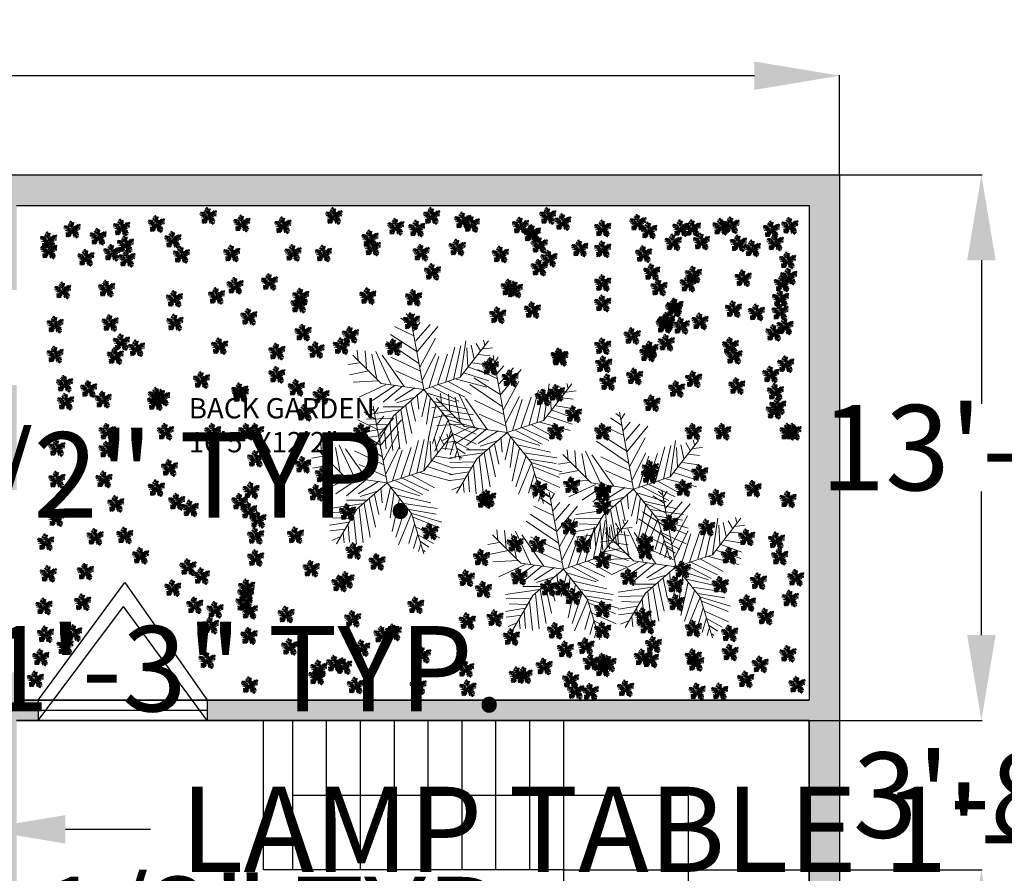
# Model space of a CAD drawing. Units: inches. Extents: x 23 to 3024, y 4 to 1405.
# Tile 6 of 7: x 2558 to 2849, y 1090 to 1342. Entities that reach past the tile are written whole.
import ezdxf

# ---------------------------------------------------------------- set-up
doc = ezdxf.new("R2010")
doc.units = ezdxf.units.IN
doc.header["$MEASUREMENT"] = 0
for name, color, linetype, lineweight in [('A-ANNO-DIMS', 2, 'Continuous', 18), ('A-DOOR', 4, 'Continuous', 25), ('A-FLOR-STRS', 7, 'Continuous', 25), ('A-WALL', 7, 'Continuous', 35), ('A-WALL-PATT', 189, 'Continuous', 13), ('C-PROP', 7, 'Continuous', 30), ('L-PLNT', 114, 'Continuous', 13)]:
    doc.layers.add(name, color=color, linetype=linetype, lineweight=lineweight)
doc.layers.add('A-AREA-IDEN', color=30, linetype='Continuous', lineweight=18, true_color=0xf8991e)
doc.styles.get("Standard").update_dxf_attribs({"font": 'arial.ttf'})
doc.dimstyles.get("Standard").update_dxf_attribs({"dimtxt": 25.18, "dimasz": 25.18, "dimexe": 0.18, "dimexo": 0.0625, "dimgap": 0.09, "dimtad": 0, "dimtih": 1, "dimtoh": 1, "dimdec": 0, "dimrnd": 10, "dimzin": 0, "dimdsep": 46, "dimlunit": 3, "dimtxsty": 'Standard', "dimcen": 0.09, "dimadec": 0, "dimazin": 0, "dimtfac": 1, "dimtdec": 0, "dimtofl": 0, "dimtmove": 0, "dimatfit": 3, "dimfxl": 1, "dimtolj": 1, "dimtzin": 0, "dimarcsym": 0})

# ---------------------------------------------------------------- blocks, each defined once
blk = doc.blocks.new('*U8')
for p, q in [((-8.737, 47.138), (-17.069, 52.711)), ((-10.186, 53.64), (-13.084, 55.962)), ((0, 0), (-10.5, 57)), ((-9.099, 51.782), (-6.563, 55.962)), ((-7.288, 39.707), (-21.778, 46.673)), ((-7.65, 43.423), (-2.578, 49.46)), ((-5.839, 35.992), (4.667, 48.067)), ((-5.114, 27.632), (10.463, 46.673)), ((-5.114, 28.097), (-24.676, 40.636)), ((-2.941, 16.486), (8.652, 37.85)), ((-3.665, 19.273), (-27.574, 35.527)), ((16.259, 5.805), (23.142, 31.348)), ((22.055, 7.198), (27.489, 32.277)), ((27, 9), (48, 36)), ((27.127, 9.056), (31.112, 35.992)), ((31.836, 30.883), (32.561, 16.486)), ((35.096, 32.741), (37.27, 22.524)), ((38.719, 34.134), (41.979, 28.561)), ((43.791, 29.954), (51.036, 30.883)), ((44.153, 36.456), (45.239, 32.741)), ((-31.5, 4.5), (-52.5, 25.5)), ((-48.585, 21.131), (-49.309, 29.026)), ((-43.513, 28.561), (-42.427, 15.558)), ((-38.442, 26.239), (-34.819, 7.663)), ((-35.544, 28.097), (-24.314, 3.947)), ((-14.533, 2.09), (-30.834, 25.31)), ((-24.314, 23.917), (-2.941, 13.7)), ((-1.129, 6.734), (9.014, 26.704)), ((3.942, 1.625), (11.187, 24.381)), ((10.101, 3.483), (17.708, 26.239)), ((40.53, 25.775), (48.862, 24.846)), ((-47.498, 19.737), (-55.83, 18.344)), ((33.285, 16.486), (48.862, 10.913)), ((36.183, 19.737), (48.137, 17.88)), ((-40.615, 13.7), (-55.105, 10.913)), ((-20.691, 13.7), (-1.129, 4.876)), ((0, 0), (27, 9)), ((24.229, 7.663), (46.688, 1.625)), ((29.662, 12.307), (48.137, 6.269)), ((-33.37, 6.269), (-52.207, 5.34)), ((-28.299, 3.483), (-47.86, -5.805)), ((-21.416, 3.018), (-38.079, -8.128)), ((0, 0), (-31.5, 4.5)), ((-15.982, 2.09), (-30.11, -9.521)), ((0, 0), (-22.5, -19.5)), ((-6.563, 1.161), (-21.416, -8.128)), ((0, 0), (18, -22.5)), ((6.478, 1.625), (26.04, -8.592)), ((11.187, 3.483), (30.749, -5.805)), ((18.07, 5.805), (35.096, -3.483)), ((-6.563, -5.805), (-19.967, -9.985)), ((-4.752, -3.483), (-3.665, -14.629)), ((2.493, -3.019), (-1.491, -20.202)), ((1.769, -2.555), (24.229, -9.521)), ((5.029, -6.27), (2.131, -25.775)), ((-15.257, -12.772), (-30.11, -12.772)), ((-13.446, -11.378), (-8.737, -32.741)), ((-9.461, -8.592), (-6.201, -23.453)), ((9.014, -11.378), (3.58, -35.992)), ((7.565, -9.056), (32.198, -14.629)), ((-17.431, -15.094), (-42.789, -18.809)), ((-24.314, -21.596), (-42.427, -22.06)), ((-22.5, -19.5), (-37.5, -45)), ((-20.691, -18.345), (-17.793, -44.352)), ((-17.069, -15.094), (-12.721, -40.172)), ((14.085, -16.951), (6.478, -40.172)), ((12.274, -15.094), (36.907, -18.809)), ((16.259, -19.738), (36.183, -22.989)), ((-28.299, -29.026), (-42.789, -31.348)), ((-26.849, -26.24), (-40.253, -25.775)), ((-25.038, -23.918), (-22.865, -45.281)), ((18.07, -22.524), (8.289, -45.745)), ((18, -22.5), (27, -52.5)), ((18.433, -22.524), (40.53, -29.026)), ((19.157, -25.311), (38.719, -33.206)), ((-30.834, -34.135), (-42.427, -35.528)), ((-29.023, -30.884), (-27.936, -43.887)), ((20.244, -30.419), (15.897, -44.816)), ((21.331, -32.741), (39.081, -40.636)), ((-34.457, -39.708), (-40.978, -42.494)), ((-32.646, -36.921), (-31.921, -44.352)), ((22.78, -37.85), (19.519, -48.532)), ((22.78, -38.314), (34.372, -44.816)), ((24.591, -43.423), (30.749, -47.603)), ((24.591, -45.745), (23.142, -50.854)), ((26.764, -49.925), (28.213, -50.854))]:
    blk.add_line(p, q)
blk = doc.blocks.new('*D9')
at = {"layer": 'A-ANNO-DIMS', "color": 0, "lineweight": -2, "transparency": 16777216}
for p, q in [((2200.45, 1295.99), (2200.45, 1325.4)), ((2225.63, 1325.22), (2478.99, 1325.22)), ((2775.27, 1325.22), (2521.91, 1325.22)), ((2800.45, 1295.99), (2800.45, 1325.4))]:
    blk.add_line(p, q, dxfattribs=at)
at = {"layer": 'A-ANNO-DIMS', "color": 0, "transparency": 16777216}
for points in [[(2225.63, 1329.42), (2225.63, 1321.02), (2200.45, 1325.22)], [(2775.27, 1329.42), (2775.27, 1321.02), (2800.45, 1325.22)]]:
    blk.add_solid(points, dxfattribs=at)
at = {"layer": 'Defpoints', "color": 0, "transparency": 16777216}
for p in [(2800.45, 1325.22), (2200.45, 1295.93), (2800.45, 1295.93)]:
    blk.add_point(p, dxfattribs=at)
at = {"layer": 'A-ANNO-DIMS', "color": 0, "transparency": 16777216, "insert": (2500.45, 1325.22), "char_height": 25.18, "attachment_point": 5}
blk.add_mtext("\\A1;50'", dxfattribs=at)
blk = doc.blocks.new('*D25')
at = {"layer": 'A-ANNO-DIMS', "color": 0, "lineweight": -2, "transparency": 16777216}
for p, q in [((2273.17, 1211.86), (2273.17, 1207.21)), ((2303.45, 1211.86), (2303.45, 1207.21)), ((2247.99, 1207.39), (2222.81, 1207.39)), ((2328.63, 1207.39), (2353.81, 1207.39))]:
    blk.add_line(p, q, dxfattribs=at)
at = {"layer": 'A-ANNO-DIMS', "color": 0, "transparency": 16777216}
for points in [[(2247.99, 1211.58), (2247.99, 1203.19), (2273.17, 1207.39)], [(2328.63, 1211.58), (2328.63, 1203.19), (2303.45, 1207.39)]]:
    blk.add_solid(points, dxfattribs=at)
at = {"layer": 'Defpoints', "color": 0, "transparency": 16777216}
for p in [(2273.17, 1211.93), (2303.45, 1211.93), (2303.45, 1207.39)]:
    blk.add_point(p, dxfattribs=at)
at = {"layer": 'A-ANNO-DIMS', "color": 0, "transparency": 16777216, "insert": (2517, 1207.39), "char_height": 25.18, "attachment_point": 5}
blk.add_mtext('\\A1;DOOR 2\'-6 1/2" TYP.', dxfattribs=at)
blk = doc.blocks.new('*D37')
at = {"layer": 'A-ANNO-DIMS', "color": 0, "lineweight": -2, "transparency": 16777216}
for p, q in [((2214.42, 1078.46), (2214.42, 1076)), ((2230.01, 1078.46), (2230.01, 1076)), ((2189.24, 1076.18), (2164.06, 1076.18)), ((2255.19, 1076.18), (2280.37, 1076.18))]:
    blk.add_line(p, q, dxfattribs=at)
at = {"layer": 'A-ANNO-DIMS', "color": 0, "transparency": 16777216}
for points in [[(2189.24, 1080.38), (2189.24, 1071.99), (2214.42, 1076.18)], [(2255.19, 1080.38), (2255.19, 1071.99), (2230.01, 1076.18)]]:
    blk.add_solid(points, dxfattribs=at)
at = {"layer": 'Defpoints', "color": 0, "transparency": 16777216}
for p in [(2214.42, 1078.52), (2230.01, 1078.52), (2230.01, 1076.18)]:
    blk.add_point(p, dxfattribs=at)
at = {"layer": 'A-ANNO-DIMS', "color": 0, "transparency": 16777216, "insert": (2499.37, 1076.18), "char_height": 25.18, "attachment_point": 5}
blk.add_mtext('\\A1;LAMP TABLE 1\'-3 1/2" TYP.', dxfattribs=at)
blk = doc.blocks.new('*D39')
at = {"layer": 'A-ANNO-DIMS', "color": 0, "lineweight": -2, "transparency": 16777216}
for p, q in [((2501.85, 1102.79), (2476.67, 1102.79)), ((2527.03, 1099.9), (2527.03, 1102.97)), ((2546.68, 1099.9), (2546.68, 1102.97)), ((2571.86, 1102.79), (2597.04, 1102.79))]:
    blk.add_line(p, q, dxfattribs=at)
at = {"layer": 'A-ANNO-DIMS', "color": 0, "transparency": 16777216}
for points in [[(2501.85, 1106.99), (2501.85, 1098.59), (2527.03, 1102.79)], [(2571.86, 1106.99), (2571.86, 1098.59), (2546.68, 1102.79)]]:
    blk.add_solid(points, dxfattribs=at)
at = {"layer": 'Defpoints', "color": 0, "transparency": 16777216}
for p in [(2546.68, 1102.79), (2527.03, 1099.84), (2546.68, 1099.84)]:
    blk.add_point(p, dxfattribs=at)
at = {"layer": 'A-ANNO-DIMS', "color": 0, "transparency": 16777216, "insert": (2816.04, 1102.79), "char_height": 25.18, "attachment_point": 5}
blk.add_mtext('\\A1;LAMP TABLE 1\'-7 1/2" TYP.', dxfattribs=at)
blk = doc.blocks.new('*D40')
at = {"layer": 'A-ANNO-DIMS', "color": 0, "lineweight": -2, "transparency": 16777216}
for p, q in [((2524.09, 1125.02), (2524.09, 1150.2)), ((2524.09, 1150.2), (2549.27, 1150.2)), ((2526.97, 1099.84), (2523.91, 1099.84)), ((2526.97, 1084.82), (2523.91, 1084.82)), ((2524.09, 1059.64), (2524.09, 1034.46))]:
    blk.add_line(p, q, dxfattribs=at)
at = {"layer": 'A-ANNO-DIMS', "color": 0, "transparency": 16777216}
for points in [[(2519.89, 1125.02), (2528.28, 1125.02), (2524.09, 1099.84)], [(2519.89, 1059.64), (2528.28, 1059.64), (2524.09, 1084.82)]]:
    blk.add_solid(points, dxfattribs=at)
at = {"layer": 'Defpoints', "color": 0, "transparency": 16777216}
for p in [(2524.09, 1099.84), (2527.03, 1099.84), (2527.03, 1084.82)]:
    blk.add_point(p, dxfattribs=at)
at = {"layer": 'A-ANNO-DIMS', "color": 0, "transparency": 16777216, "insert": (2624.91, 1150.2), "char_height": 25.18, "attachment_point": 5}
blk.add_mtext('\\A1;1\'-3" TYP.', dxfattribs=at)
blk = doc.blocks.new('*D43')
at = {"layer": 'A-ANNO-DIMS', "color": 0, "lineweight": -2, "transparency": 16777216}
for p, q in [((2800.51, 1295.93), (2842.48, 1295.93)), ((2842.3, 1270.75), (2842.3, 1228.38)), ((2842.3, 1160.11), (2842.3, 1202.47)), ((2791.51, 1134.93), (2842.48, 1134.93))]:
    blk.add_line(p, q, dxfattribs=at)
at = {"layer": 'A-ANNO-DIMS', "color": 0, "transparency": 16777216}
for points in [[(2838.1, 1270.75), (2846.5, 1270.75), (2842.3, 1295.93)], [(2838.1, 1160.11), (2846.5, 1160.11), (2842.3, 1134.93)]]:
    blk.add_solid(points, dxfattribs=at)
at = {"layer": 'Defpoints', "color": 0, "transparency": 16777216}
for p in [(2800.45, 1295.93), (2791.45, 1134.93), (2842.3, 1134.93)]:
    blk.add_point(p, dxfattribs=at)
at = {"layer": 'A-ANNO-DIMS', "color": 0, "transparency": 16777216, "insert": (2842.3, 1215.43), "char_height": 25.18, "attachment_point": 5}
blk.add_mtext('\\A1;13\'-5"', dxfattribs=at)
blk = doc.blocks.new('*D46')
at = {"layer": 'A-ANNO-DIMS', "color": 0, "lineweight": -2, "transparency": 16777216}
for p, q in [((2719.07, 1090.84), (2842.48, 1090.84)), ((2842.3, 1065.66), (2842.3, 1052.75)), ((2842.3, 1013.96), (2842.3, 1026.86)), ((2791.51, 988.78), (2842.48, 988.78))]:
    blk.add_line(p, q, dxfattribs=at)
at = {"layer": 'A-ANNO-DIMS', "color": 0, "transparency": 16777216}
for points in [[(2838.1, 1065.66), (2846.5, 1065.66), (2842.3, 1090.84)], [(2838.1, 1013.96), (2846.5, 1013.96), (2842.3, 988.78)]]:
    blk.add_solid(points, dxfattribs=at)
at = {"layer": 'Defpoints', "color": 0, "transparency": 16777216}
for p in [(2719, 1090.84), (2842.3, 1090.84), (2791.45, 988.78)]:
    blk.add_point(p, dxfattribs=at)
at = {"layer": 'A-ANNO-DIMS', "color": 0, "transparency": 16777216, "insert": (2842.3, 1039.81), "char_height": 25.18, "attachment_point": 5}
blk.add_mtext('\\A1;8\'-6"', dxfattribs=at)
blk = doc.blocks.new('*D47')
at = {"layer": 'A-ANNO-DIMS', "color": 0, "lineweight": -2, "transparency": 16777216}
for p, q in [((2842.3, 1160.11), (2842.3, 1185.29)), ((2719.07, 1134.93), (2842.48, 1134.93)), ((2719.07, 1090.84), (2842.48, 1090.84)), ((2842.3, 1065.66), (2842.3, 1040.48))]:
    blk.add_line(p, q, dxfattribs=at)
at = {"layer": 'A-ANNO-DIMS', "color": 0, "transparency": 16777216}
for points in [[(2838.1, 1160.11), (2846.5, 1160.11), (2842.3, 1134.93)], [(2838.1, 1065.66), (2846.5, 1065.66), (2842.3, 1090.84)]]:
    blk.add_solid(points, dxfattribs=at)
at = {"layer": 'Defpoints', "color": 0, "transparency": 16777216}
for p in [(2719, 1134.93), (2842.3, 1134.93), (2719, 1090.84)]:
    blk.add_point(p, dxfattribs=at)
at = {"layer": 'A-ANNO-DIMS', "color": 0, "transparency": 16777216, "insert": (2842.3, 1112.88), "char_height": 25.18, "attachment_point": 5}
blk.add_mtext('\\A1;3\'-8"', dxfattribs=at)

msp = doc.modelspace()

# ---------------------------------------------------------------- hatches: boundary and pattern name
at = {"layer": 'A-WALL-PATT'}
h = msp.add_hatch(color=256, dxfattribs=at)
h.dxf.hatch_style = 1
h.paths.add_polyline_path([(2209.45, 1233.93), (2200.45, 1233.93), (2200.45, 1160.43), (2209.45, 1160.43), (2209.45, 1167.77), (2209.45, 1202.93), (2306.45, 1202.93), (2306.45, 1208.93), (2300.45, 1208.93), (2209.45, 1208.93)], flags=17)
h.paths.add_polyline_path([(2800.45, 1295.93), (2200.45, 1295.93), (2160.45, 1295.93), (2160.45, 575.93), (2200.45, 575.93), (2228.06, 575.93), (2228.06, 584.93), (2209.45, 584.93), (2209.45, 856.93), (2200.45, 856.93), (2200.45, 581.93), (2166.45, 581.93), (2166.45, 1289.93), (2200.45, 1289.93), (2200.45, 1261.93), (2209.45, 1261.93), (2209.45, 1286.93), (2244.45, 1286.93), (2300.45, 1286.93), (2300.45, 1241.93), (2301.45, 1241.93, -0.017236), (2303.45, 1241.93), (2306.45, 1241.93), (2306.45, 1286.93), (2548.45, 1286.93), (2548.45, 1261.93), (2557.45, 1261.93), (2557.45, 1286.93), (2791.45, 1286.93), (2791.45, 1140.93), (2613.74, 1140.93), (2613.74, 1134.93), (2791.45, 1134.93), (2791.45, 927.1), (2800.45, 927.1)])
h.paths.add_polyline_path([(2166.06, 1284.53), (2166.03, 1284.87), (2166.29, 1284.91), (2166.32, 1284.58)], flags=16)
h.paths.add_polyline_path([(2557.45, 1233.93), (2548.45, 1233.93), (2548.45, 1208.93), (2514.78, 1208.93), (2457.45, 1208.93), (2451.45, 1208.93), (2451.45, 1202.93), (2548.45, 1202.93), (2557.45, 1202.93)], flags=17)
h.paths.add_polyline_path([(2457.45, 1286.93), (2451.45, 1286.93), (2451.45, 1241.93), (2454.45, 1241.93, -0.017236), (2456.45, 1241.93), (2457.45, 1241.93)], flags=17)
h.paths.add_polyline_path([(2419.96, 1208.93), (2378.45, 1208.93), (2378.45, 1286.93), (2372.45, 1286.93), (2372.45, 1208.93), (2352.45, 1208.93), (2352.45, 1202.93), (2419.96, 1202.93)], flags=17)
h.paths.add_polyline_path([(2557.45, 1134.93), (2563.84, 1134.93), (2563.84, 1140.93), (2557.45, 1140.93), (2557.45, 1149.12), (2548.45, 1149.12), (2548.45, 1103.07), (2548.45, 1065.93), (2416.45, 1065.93), (2416.45, 1064.93, -0.014283), (2416.45, 1062.93), (2416.45, 1059.93), (2548.45, 1059.93), (2548.45, 1025.12), (2557.45, 1025.12)], flags=17)
h.paths.add_polyline_path([(2332.45, 1062.93, -0.014283), (2332.45, 1064.93), (2332.45, 1065.93), (2209.45, 1065.93), (2209.45, 1108.43), (2200.45, 1108.43), (2200.45, 1042.43), (2209.45, 1042.43), (2209.45, 1059.93), (2332.45, 1059.93)], flags=17)
h.paths.add_polyline_path([(2332.45, 996.93), (2209.45, 996.93), (2209.45, 1014.43), (2200.45, 1014.43), (2200.45, 952.93), (2209.45, 952.93), (2209.45, 990.93), (2332.45, 990.93), (2332.45, 991.93, -0.014283), (2332.45, 993.93)], flags=17)
h.paths.add_polyline_path([(2209.45, 900.93), (2200.45, 900.93), (2200.45, 856.93), (2209.45, 856.93), (2255.95, 856.93), (2255.95, 862.93), (2209.45, 862.93)], flags=17)
h.paths.add_polyline_path([(2377.45, 823.93), (2374.45, 823.93, -0.017236), (2372.45, 823.93), (2371.45, 823.93), (2371.45, 763.93), (2312.45, 763.93), (2312.45, 791.27), (2312.45, 796.43), (2306.45, 796.43), (2306.45, 757.93), (2436.95, 757.93), (2436.95, 763.93), (2377.45, 763.93)], flags=17)
h.paths.add_polyline_path([(2557.45, 948.81), (2548.45, 948.81), (2548.45, 763.93), (2488.95, 763.93), (2488.95, 757.93), (2560.45, 757.93), (2560.45, 760.93), (2562.45, 760.93), (2562.45, 763.93), (2557.45, 763.93)], flags=17)
h.paths.add_polyline_path([(2377.45, 990.93), (2371.45, 990.93), (2371.45, 862.93), (2306.45, 862.93), (2306.45, 856.93), (2306.45, 824.43), (2312.45, 824.43), (2312.45, 856.93), (2371.45, 856.93), (2377.45, 856.93)], flags=17)
h.paths.add_polyline_path([(2800.45, 875.1), (2791.45, 875.1), (2791.45, 763.93), (2719.93, 763.93), (2719.93, 757.93), (2791.45, 757.93), (2791.45, 584.93), (2338.88, 584.93), (2338.88, 575.93), (2800.45, 575.93)], flags=17)
h.paths.add_polyline_path([(2667.93, 763.93), (2596.45, 763.93), (2596.45, 762.93, -0.014283), (2596.45, 760.93), (2596.45, 757.93), (2667.93, 757.93)], flags=16)

# ---------------------------------------------------------------- linework, layer by layer
at = {"layer": 'A-DOOR'}
for p, q in [((2563.84, 1140.93), (2589.4, 1175.61)), ((2589.4, 1175.61), (2613.74, 1140.93)), ((2563.84, 1134.93), (2589, 1168.58)), ((2613.74, 1134.93), (2589, 1168.58)), ((2563.84, 1140.93), (2563.84, 1134.93)), ((2613.74, 1140.93), (2613.74, 1134.93)), ((2563.84, 1137.93), (2613.74, 1137.93))]:
    msp.add_line(p, q, dxfattribs=at)
at = {"layer": 'A-FLOR-STRS'}
for p, q in [((2630.35, 1090.84), (2630.35, 1134.93)), ((2639, 1090.84), (2639, 1134.93)), ((2649, 1090.84), (2649, 1134.93)), ((2659, 1090.84), (2659, 1134.93)), ((2669, 1090.84), (2669, 1134.93)), ((2679, 1090.84), (2679, 1134.93)), ((2689, 1090.84), (2689, 1134.93)), ((2699, 1090.84), (2699, 1134.93)), ((2709, 1090.84), (2709, 1134.93)), ((2719, 1090.84), (2719, 1134.93)), ((2639, 1112.88), (2755.69, 1112.88)), ((2755.69, 1112.88), (2755.69, 1038.78)), ((2719, 1090.84), (2630.35, 1090.84)), ((2719, 988.78), (2719, 1090.84))]:
    msp.add_line(p, q, dxfattribs=at)
at = {"layer": 'A-WALL'}
for p, q in [((2557.45, 1140.93), (2791.45, 1140.93)), ((2557.45, 1134.93), (2791.45, 1134.93)), ((2791.45, 1134.93), (2791.45, 763.93))]:
    msp.add_line(p, q, dxfattribs=at)
at = {"layer": 'C-PROP'}
for p, q in [((2200.45, 1295.93), (2800.45, 1295.93)), ((2800.45, 1295.93), (2800.45, 575.93)), ((2557.45, 1286.93), (2791.45, 1286.93)), ((2791.45, 1286.93), (2791.45, 1140.93))]:
    msp.add_line(p, q, dxfattribs=at)

# ---------------------------------------------------------------- block references
at = {"layer": 'L-PLNT'}
for p, xscale, yscale, zscale in [((2614.18, 1283.71), 0.0466330202614855, 0.0466330202614855, 0.0466330202614855), ((2651.27, 1283.71), 0.0466330202614855, 0.0466330202614855, 0.0466330202614855), ((2680.12, 1283.71), 0.0466330202614855, 0.0466330202614855, 0.0466330202614855), ((2689.31, 1282.38), 0.0466330202614855, 0.0466330202614855, 0.0466330202614855), ((2714.43, 1283.71), 0.0466330202614855, 0.0466330202614855, 0.0466330202614855), ((2574, 1279.68), 0.0466330202614855, 0.0466330202614855, 0.0466330202614855), ((2588.58, 1280.29), 0.0466330202614855, 0.0466330202614855, 0.0466330202614855), ((2598.85, 1281.34), 0.0466330202614855, 0.0466330202614855, 0.0466330202614855), ((2624.1, 1281.52), 0.0466330202614855, 0.0466330202614855, 0.0466330202614855), ((2636.22, 1280.96), 0.0466330202614855, 0.0466330202614855, 0.0466330202614855), ((2669.56, 1280.54), 0.0466330202614855, 0.0466330202614855, 0.0466330202614855), ((2675.73, 1280.02), 0.0466330202614855, 0.0466330202614855, 0.0466330202614855), ((2691.85, 1281.34), 0.0466330202614855, 0.0466330202614855, 0.0466330202614855), ((2706.35, 1280.88), 0.0466330202614855, 0.0466330202614855, 0.0466330202614855), ((2718.86, 1281.93), 0.0466330202614855, 0.0466330202614855, 0.0466330202614855), ((2730.61, 1280.04), 0.0466330202614855, 0.0466330202614855, 0.0466330202614855), ((2741.01, 1281.72), 0.0466330202614855, 0.0466330202614855, 0.0466330202614855), ((2744.21, 1279.42), 0.0466330202614855, 0.0466330202614855, 0.0466330202614855), ((2753.69, 1280.12), 0.0466330202614855, 0.0466330202614855, 0.0466330202614855), ((2757.09, 1280.12), 0.0466330202614855, 0.0466330202614855, 0.0466330202614855), ((2765.54, 1280.52), 0.0466330202614855, 0.0466330202614855, 0.0466330202614855), ((2768.5, 1280.97), 0.0466330202614855, 0.0466330202614855, 0.0466330202614855), ((2780.43, 1279.76), 0.0466330202614855, 0.0466330202614855, 0.0466330202614855), ((2785.88, 1280.8), 0.0466330202614855, 0.0466330202614855, 0.0466330202614855), ((2567.02, 1276.53), 0.0466330202614855, 0.0466330202614855, 0.0466330202614855), ((2581.67, 1277.57), 0.0466330202614855, 0.0466330202614855, 0.0466330202614855), ((2603.73, 1276.69), 0.0466330202614855, 0.0466330202614855, 0.0466330202614855), ((2661.94, 1277.1), 0.0466330202614855, 0.0466330202614855, 0.0466330202614855), ((2709.55, 1278.53), 0.0466330202614855, 0.0466330202614855, 0.0466330202614855), ((2709.86, 1278.65), 0.0466330202614855, 0.0466330202614855, 0.0466330202614855), ((2567.1, 1273.53), 0.0466330202614855, 0.0466330202614855, 0.0466330202614855), ((2589.74, 1275.36), 0.0466330202614855, 0.0466330202614855, 0.0466330202614855), ((2662.61, 1274.39), 0.0466330202614855, 0.0466330202614855, 0.0466330202614855), ((2687.67, 1274.39), 0.0466330202614855, 0.0466330202614855, 0.0466330202614855), ((2711.9, 1275.17), 0.0466330202614855, 0.0466330202614855, 0.0466330202614855), ((2723.86, 1274.14), 0.0466330202614855, 0.0466330202614855, 0.0466330202614855), ((2730.61, 1273.88), 0.0466330202614855, 0.0466330202614855, 0.0466330202614855), ((2751.44, 1275.91), 0.0466330202614855, 0.0466330202614855, 0.0466330202614855), ((2759.79, 1276.16), 0.0466330202614855, 0.0466330202614855, 0.0466330202614855), ((2770.68, 1275.65), 0.0466330202614855, 0.0466330202614855, 0.0466330202614855), ((2774.79, 1274.13), 0.0466330202614855, 0.0466330202614855, 0.0466330202614855), ((2781.56, 1275.91), 0.0466330202614855, 0.0466330202614855, 0.0466330202614855), ((2578.07, 1271.36), 0.0466330202614855, 0.0466330202614855, 0.0466330202614855), ((2585.72, 1272.88), 0.0466330202614855, 0.0466330202614855, 0.0466330202614855), ((2590.15, 1271.1), 0.0466330202614855, 0.0466330202614855, 0.0466330202614855), ((2606.25, 1272.24), 0.0466330202614855, 0.0466330202614855, 0.0466330202614855), ((2621.11, 1272.62), 0.0466330202614855, 0.0466330202614855, 0.0466330202614855), ((2639.19, 1272.81), 0.0466330202614855, 0.0466330202614855, 0.0466330202614855), ((2648.19, 1272.62), 0.0466330202614855, 0.0466330202614855, 0.0466330202614855), ((2677.04, 1272.87), 0.0466330202614855, 0.0466330202614855, 0.0466330202614855), ((2700.41, 1272.34), 0.0466330202614855, 0.0466330202614855, 0.0466330202614855), ((2714.75, 1271.1), 0.0466330202614855, 0.0466330202614855, 0.0466330202614855), ((2742.69, 1272.48), 0.0466330202614855, 0.0466330202614855, 0.0466330202614855), ((2785.21, 1270.6), 0.0466330202614855, 0.0466330202614855, 0.0466330202614855), ((2711.9, 1268.45), 0.0466330202614855, 0.0466330202614855, 0.0466330202614855), ((2680.35, 1267.2), 0.0466330202614855, 0.0466330202614855, 0.0466330202614855), ((2745.13, 1267.13), 0.0466330202614855, 0.0466330202614855, 0.0466330202614855), ((2757.4, 1266.42), 0.0466330202614855, 0.0466330202614855, 0.0466330202614855), ((2772.08, 1265.32), 0.0466330202614855, 0.0466330202614855, 0.0466330202614855), ((2785.53, 1265.83), 0.0466330202614855, 0.0466330202614855, 0.0466330202614855), ((2584.16, 1262.26), 0.0466330202614855, 0.0466330202614855, 0.0466330202614855), ((2622.09, 1263.12), 0.0466330202614855, 0.0466330202614855, 0.0466330202614855), ((2632.23, 1264.22), 0.0466330202614855, 0.0466330202614855, 0.0466330202614855), ((2702.99, 1262.57), 0.0466330202614855, 0.0466330202614855, 0.0466330202614855), ((2704.55, 1262), 0.0466330202614855, 0.0466330202614855, 0.0466330202614855), ((2730.61, 1263.9), 0.0466330202614855, 0.0466330202614855, 0.0466330202614855), ((2747.23, 1262.57), 0.0466330202614855, 0.0466330202614855, 0.0466330202614855), ((2755.83, 1263.71), 0.0466330202614855, 0.0466330202614855, 0.0466330202614855), ((2783.66, 1263.79), 0.0466330202614855, 0.0466330202614855, 0.0466330202614855), ((2571.25, 1261.75), 0.0466330202614855, 0.0466330202614855, 0.0466330202614855), ((2604.19, 1259.25), 0.0466330202614855, 0.0466330202614855, 0.0466330202614855), ((2616.61, 1260.11), 0.0466330202614855, 0.0466330202614855, 0.0466330202614855), ((2641.48, 1259.91), 0.0466330202614855, 0.0466330202614855, 0.0466330202614855), ((2661.27, 1260.06), 0.0466330202614855, 0.0466330202614855, 0.0466330202614855), ((2674.79, 1259.56), 0.0466330202614855, 0.0466330202614855, 0.0466330202614855), ((2783.15, 1259.37), 0.0466330202614855, 0.0466330202614855, 0.0466330202614855), ((2640.93, 1257.54), 0.0466330202614855, 0.0466330202614855, 0.0466330202614855), ((2730.61, 1257.91), 0.0466330202614855, 0.0466330202614855, 0.0466330202614855), ((2751.58, 1256.35), 0.0466330202614855, 0.0466330202614855, 0.0466330202614855), ((2751.95, 1256.98), 0.0466330202614855, 0.0466330202614855, 0.0466330202614855), ((2769.23, 1256.19), 0.0466330202614855, 0.0466330202614855, 0.0466330202614855), ((2626.16, 1253.92), 0.0466330202614855, 0.0466330202614855, 0.0466330202614855), ((2699.62, 1254.4), 0.0466330202614855, 0.0466330202614855, 0.0466330202614855), ((2709.88, 1255.94), 0.0466330202614855, 0.0466330202614855, 0.0466330202614855), ((2776, 1255.25), 0.0466330202614855, 0.0466330202614855, 0.0466330202614855), ((2782.98, 1255.46), 0.0466330202614855, 0.0466330202614855, 0.0466330202614855), ((2568.97, 1251.64), 0.0466330202614855, 0.0466330202614855, 0.0466330202614855), ((2585.22, 1252.12), 0.0466330202614855, 0.0466330202614855, 0.0466330202614855), ((2604.34, 1252.25), 0.0466330202614855, 0.0466330202614855, 0.0466330202614855), ((2677.67, 1232.62), 0.3984345914112191, 0.3984345914112191, 0.3984345914112191), ((2674.14, 1252.63), 0.0466330202614855, 0.0466330202614855, 0.0466330202614855), ((2748.83, 1251.57), 0.0466330202614855, 0.0466330202614855, 0.0466330202614855), ((2749.17, 1252.17), 0.0466330202614855, 0.0466330202614855, 0.0466330202614855), ((2749.53, 1252.79), 0.0466330202614855, 0.0466330202614855, 0.0466330202614855), ((2753.82, 1251.25), 0.0466330202614855, 0.0466330202614855, 0.0466330202614855), ((2759.35, 1252.59), 0.0466330202614855, 0.0466330202614855, 0.0466330202614855), ((2784.46, 1251.11), 0.0466330202614855, 0.0466330202614855, 0.0466330202614855), ((2642.15, 1249.27), 0.0466330202614855, 0.0466330202614855, 0.0466330202614855), ((2656.13, 1248.6), 0.0466330202614855, 0.0466330202614855, 0.0466330202614855), ((2739.33, 1248.29), 0.0466330202614855, 0.0466330202614855, 0.0466330202614855), ((2781.18, 1249.22), 0.0466330202614855, 0.0466330202614855, 0.0466330202614855), ((2588.53, 1246.45), 0.0466330202614855, 0.0466330202614855, 0.0466330202614855), ((2592.96, 1244.67), 0.0466330202614855, 0.0466330202614855, 0.0466330202614855), ((2617.51, 1245.28), 0.0466330202614855, 0.0466330202614855, 0.0466330202614855), ((2653.47, 1245.28), 0.0466330202614855, 0.0466330202614855, 0.0466330202614855), ((2668.93, 1244.95), 0.0466330202614855, 0.0466330202614855, 0.0466330202614855), ((2730.61, 1245.26), 0.0466330202614855, 0.0466330202614855, 0.0466330202614855), ((2749.39, 1246.29), 0.0466330202614855, 0.0466330202614855, 0.0466330202614855), ((2768.33, 1245.42), 0.0466330202614855, 0.0466330202614855, 0.0466330202614855), ((2568.97, 1242.79), 0.0466330202614855, 0.0466330202614855, 0.0466330202614855), ((2586.73, 1242.37), 0.0466330202614855, 0.0466330202614855, 0.0466330202614855), ((2634.43, 1243.68), 0.0466330202614855, 0.0466330202614855, 0.0466330202614855), ((2646.02, 1244.15), 0.0466330202614855, 0.0466330202614855, 0.0466330202614855), ((2717.78, 1242.25), 0.0466330202614855, 0.0466330202614855, 0.0466330202614855), ((2717.99, 1241.88), 0.0466330202614855, 0.0466330202614855, 0.0466330202614855), ((2743.95, 1243.13), 0.0466330202614855, 0.0466330202614855, 0.0466330202614855), ((2744.63, 1244.3), 0.0466330202614855, 0.0466330202614855, 0.0466330202614855), ((2769.37, 1242.4), 0.0466330202614855, 0.0466330202614855, 0.0466330202614855), ((2702.3, 1219.89), 0.3984345914112191, 0.3984345914112191, 0.3984345914112191), ((2697.45, 1239.17), 0.0466330202614855, 0.0466330202614855, 0.0466330202614855), ((2730.91, 1239.94), 0.0466330202614855, 0.0466330202614855, 0.0466330202614855), ((2784.66, 1239.96), 0.0466330202614855, 0.0466330202614855, 0.0466330202614855), ((2634.43, 1236.83), 0.0466330202614855, 0.0466330202614855, 0.0466330202614855), ((2703.31, 1235.79), 0.0466330202614855, 0.0466330202614855, 0.0466330202614855), ((2740.03, 1236.34), 0.0466330202614855, 0.0466330202614855, 0.0466330202614855), ((2780.25, 1236.92), 0.0466330202614855, 0.0466330202614855, 0.0466330202614855), ((2571.76, 1234.2), 0.0466330202614855, 0.0466330202614855, 0.0466330202614855), ((2612.18, 1235.3), 0.0466330202614855, 0.0466330202614855, 0.0466330202614855), ((2640.18, 1233), 0.0466330202614855, 0.0466330202614855, 0.0466330202614855), ((2732.13, 1234.65), 0.0466330202614855, 0.0466330202614855, 0.0466330202614855), ((2757.44, 1235.51), 0.0466330202614855, 0.0466330202614855, 0.0466330202614855), ((2770.21, 1233.51), 0.0466330202614855, 0.0466330202614855, 0.0466330202614855), ((2578.88, 1232.64), 0.0466330202614855, 0.0466330202614855, 0.0466330202614855), ((2598.86, 1230.65), 0.0466330202614855, 0.0466330202614855, 0.0466330202614855), ((2600.42, 1230.08), 0.0466330202614855, 0.0466330202614855, 0.0466330202614855), ((2623.5, 1231.98), 0.0466330202614855, 0.0466330202614855, 0.0466330202614855), ((2623.65, 1231.15), 0.0466330202614855, 0.0466330202614855, 0.0466330202614855), ((2647.47, 1230.65), 0.0466330202614855, 0.0466330202614855, 0.0466330202614855), ((2713.11, 1230.13), 0.0466330202614855, 0.0466330202614855, 0.0466330202614855), ((2716.96, 1231.49), 0.0466330202614855, 0.0466330202614855, 0.0466330202614855), ((2752.44, 1232.63), 0.0466330202614855, 0.0466330202614855, 0.0466330202614855), ((2781.62, 1231.81), 0.0466330202614855, 0.0466330202614855, 0.0466330202614855), ((2572.06, 1228.88), 0.0466330202614855, 0.0466330202614855, 0.0466330202614855), ((2583.11, 1229.5), 0.0466330202614855, 0.0466330202614855, 0.0466330202614855), ((2598.61, 1228.78), 0.0466330202614855, 0.0466330202614855, 0.0466330202614855), ((2745.16, 1228.42), 0.0466330202614855, 0.0466330202614855, 0.0466330202614855), ((2782.31, 1227.56), 0.0466330202614855, 0.0466330202614855, 0.0466330202614855), ((2642.65, 1225.61), 0.0466330202614855, 0.0466330202614855, 0.0466330202614855), ((2666.89, 1205.01), 0.3984345914112191, 0.3984345914112191, 0.3984345914112191), ((2722.01, 1225.24), 0.0466330202614855, 0.0466330202614855, 0.0466330202614855), ((2781.28, 1226.2), 0.0466330202614855, 0.0466330202614855, 0.0466330202614855), ((2739.62, 1203.22), 0.3984345914112191, 0.3984345914112191, 0.3984345914112191), ((2584.34, 1220.03), 0.0466330202614855, 0.0466330202614855, 0.0466330202614855), ((2601.52, 1220.03), 0.0466330202614855, 0.0466330202614855, 0.0466330202614855), ((2615.51, 1220.03), 0.0466330202614855, 0.0466330202614855, 0.0466330202614855), ((2625.5, 1220.03), 0.0466330202614855, 0.0466330202614855, 0.0466330202614855), ((2628.16, 1220.03), 0.0466330202614855, 0.0466330202614855, 0.0466330202614855), ((2659.46, 1220.03), 0.0466330202614855, 0.0466330202614855, 0.0466330202614855), ((2716.73, 1220.03), 0.0466330202614855, 0.0466330202614855, 0.0466330202614855), ((2730.61, 1220.03), 0.0466330202614855, 0.0466330202614855, 0.0466330202614855), ((2757.36, 1220.03), 0.0466330202614855, 0.0466330202614855, 0.0466330202614855), ((2766.01, 1220.03), 0.0466330202614855, 0.0466330202614855, 0.0466330202614855), ((2785.33, 1220.03), 0.0466330202614855, 0.0466330202614855, 0.0466330202614855), ((2786.81, 1220.03), 0.0466330202614855, 0.0466330202614855, 0.0466330202614855), ((2569.48, 1215.24), 0.0466330202614855, 0.0466330202614855, 0.0466330202614855), ((2584.27, 1214.74), 0.0466330202614855, 0.0466330202614855, 0.0466330202614855), ((2628.16, 1212.02), 0.0466330202614855, 0.0466330202614855, 0.0466330202614855), ((2642.1, 1210.27), 0.0466330202614855, 0.0466330202614855, 0.0466330202614855), ((2602.73, 1209.34), 0.0466330202614855, 0.0466330202614855, 0.0466330202614855), ((2648.14, 1207.37), 0.0466330202614855, 0.0466330202614855, 0.0466330202614855), ((2744.43, 1207.22), 0.0466330202614855, 0.0466330202614855, 0.0466330202614855), ((2744.68, 1209.08), 0.0466330202614855, 0.0466330202614855, 0.0466330202614855), ((2759.28, 1207.86), 0.0466330202614855, 0.0466330202614855, 0.0466330202614855), ((2569.48, 1205.89), 0.0466330202614855, 0.0466330202614855, 0.0466330202614855), ((2583.39, 1205.94), 0.0466330202614855, 0.0466330202614855, 0.0466330202614855), ((2721.48, 1204.22), 0.0466330202614855, 0.0466330202614855, 0.0466330202614855), ((2598.86, 1203.38), 0.0466330202614855, 0.0466330202614855, 0.0466330202614855), ((2626.83, 1202.71), 0.0466330202614855, 0.0466330202614855, 0.0466330202614855), ((2646.14, 1202.04), 0.0466330202614855, 0.0466330202614855, 0.0466330202614855), ((2711.74, 1203.16), 0.0466330202614855, 0.0466330202614855, 0.0466330202614855), ((2730.61, 1202.61), 0.0466330202614855, 0.0466330202614855, 0.0466330202614855), ((2730.61, 1202), 0.0466330202614855, 0.0466330202614855, 0.0466330202614855), ((2754.43, 1203.41), 0.0466330202614855, 0.0466330202614855, 0.0466330202614855), ((2775.02, 1203.19), 0.0466330202614855, 0.0466330202614855, 0.0466330202614855), ((2586.87, 1198.72), 0.0466330202614855, 0.0466330202614855, 0.0466330202614855), ((2604.85, 1199.38), 0.0466330202614855, 0.0466330202614855, 0.0466330202614855), ((2623.5, 1199.38), 0.0466330202614855, 0.0466330202614855, 0.0466330202614855), ((2695.72, 1199.88), 0.0466330202614855, 0.0466330202614855, 0.0466330202614855), ((2696.65, 1200.42), 0.0466330202614855, 0.0466330202614855, 0.0466330202614855), ((2718.88, 1179.59), 0.3984345914112191, 0.3984345914112191, 0.3984345914112191), ((2730.61, 1198.05), 0.0466330202614855, 0.0466330202614855, 0.0466330202614855), ((2752.11, 1180.26), 0.3984345914112191, 0.3984345914112191, 0.3984345914112191), ((2764.26, 1200.6), 0.0466330202614855, 0.0466330202614855, 0.0466330202614855), ((2785.33, 1200.05), 0.0466330202614855, 0.0466330202614855, 0.0466330202614855), ((2608.85, 1197.39), 0.0466330202614855, 0.0466330202614855, 0.0466330202614855), ((2626.16, 1196.72), 0.0466330202614855, 0.0466330202614855, 0.0466330202614855), ((2655.26, 1196.31), 0.0466330202614855, 0.0466330202614855, 0.0466330202614855), ((2569.23, 1194.52), 0.0466330202614855, 0.0466330202614855, 0.0466330202614855), ((2628.83, 1194.06), 0.0466330202614855, 0.0466330202614855, 0.0466330202614855), ((2750.39, 1193.02), 0.0466330202614855, 0.0466330202614855, 0.0466330202614855), ((2589.54, 1189.41), 0.0466330202614855, 0.0466330202614855, 0.0466330202614855), ((2628.14, 1189.28), 0.0466330202614855, 0.0466330202614855, 0.0466330202614855), ((2639.91, 1189.47), 0.0466330202614855, 0.0466330202614855, 0.0466330202614855), ((2679.61, 1190.58), 0.0466330202614855, 0.0466330202614855, 0.0466330202614855), ((2720.8, 1192), 0.0466330202614855, 0.0466330202614855, 0.0466330202614855), ((2761.31, 1191.74), 0.0466330202614855, 0.0466330202614855, 0.0466330202614855), ((2566.19, 1187.44), 0.0466330202614855, 0.0466330202614855, 0.0466330202614855), ((2580.78, 1189), 0.0466330202614855, 0.0466330202614855, 0.0466330202614855), ((2704.74, 1186.93), 0.0466330202614855, 0.0466330202614855, 0.0466330202614855), ((2711.39, 1186.73), 0.0466330202614855, 0.0466330202614855, 0.0466330202614855), ((2724.75, 1186.65), 0.0466330202614855, 0.0466330202614855, 0.0466330202614855), ((2742.99, 1187.55), 0.0466330202614855, 0.0466330202614855, 0.0466330202614855), ((2773.12, 1188.86), 0.0466330202614855, 0.0466330202614855, 0.0466330202614855), ((2781.94, 1187.99), 0.0466330202614855, 0.0466330202614855, 0.0466330202614855), ((2594.2, 1183.42), 0.0466330202614855, 0.0466330202614855, 0.0466330202614855), ((2657.18, 1184.81), 0.0466330202614855, 0.0466330202614855, 0.0466330202614855), ((2743.21, 1184.81), 0.0466330202614855, 0.0466330202614855, 0.0466330202614855), ((2768.01, 1183.42), 0.0466330202614855, 0.0466330202614855, 0.0466330202614855), ((2628.16, 1182.76), 0.0466330202614855, 0.0466330202614855, 0.0466330202614855), ((2664.01, 1181.58), 0.0466330202614855, 0.0466330202614855, 0.0466330202614855), ((2694.83, 1182.88), 0.0466330202614855, 0.0466330202614855, 0.0466330202614855), ((2730.61, 1182.09), 0.0466330202614855, 0.0466330202614855, 0.0466330202614855), ((2782.87, 1183.16), 0.0466330202614855, 0.0466330202614855, 0.0466330202614855), ((2566.95, 1178.09), 0.0466330202614855, 0.0466330202614855, 0.0466330202614855), ((2577.9, 1178.73), 0.0466330202614855, 0.0466330202614855, 0.0466330202614855), ((2608.18, 1180.1), 0.0466330202614855, 0.0466330202614855, 0.0466330202614855), ((2644.57, 1179.61), 0.0466330202614855, 0.0466330202614855, 0.0466330202614855), ((2754.1, 1179.34), 0.0466330202614855, 0.0466330202614855, 0.0466330202614855), ((2612.18, 1177.44), 0.0466330202614855, 0.0466330202614855, 0.0466330202614855), ((2653.02, 1175.23), 0.0466330202614855, 0.0466330202614855, 0.0466330202614855), ((2654.83, 1176.27), 0.0466330202614855, 0.0466330202614855, 0.0466330202614855), ((2690.36, 1176.79), 0.0466330202614855, 0.0466330202614855, 0.0466330202614855), ((2705.91, 1177.25), 0.0466330202614855, 0.0466330202614855, 0.0466330202614855), ((2738.33, 1177.14), 0.0466330202614855, 0.0466330202614855, 0.0466330202614855), ((2752.02, 1174.94), 0.0466330202614855, 0.0466330202614855, 0.0466330202614855), ((2765.33, 1174.86), 0.0466330202614855, 0.0466330202614855, 0.0466330202614855), ((2776.58, 1175.9), 0.0466330202614855, 0.0466330202614855, 0.0466330202614855), ((2787.63, 1176.93), 0.0466330202614855, 0.0466330202614855, 0.0466330202614855), ((2603.72, 1173.88), 0.0466330202614855, 0.0466330202614855, 0.0466330202614855), ((2625.25, 1172.24), 0.0466330202614855, 0.0466330202614855, 0.0466330202614855), ((2625.5, 1174.11), 0.0466330202614855, 0.0466330202614855, 0.0466330202614855), ((2695.42, 1173.44), 0.0466330202614855, 0.0466330202614855, 0.0466330202614855), ((2714.6, 1173.98), 0.0466330202614855, 0.0466330202614855, 0.0466330202614855), ((2718.55, 1173.98), 0.0466330202614855, 0.0466330202614855, 0.0466330202614855), ((2577.08, 1169.7), 0.0466330202614855, 0.0466330202614855, 0.0466330202614855), ((2610.18, 1168.79), 0.0466330202614855, 0.0466330202614855, 0.0466330202614855), ((2624.73, 1169.53), 0.0466330202614855, 0.0466330202614855, 0.0466330202614855), ((2675.44, 1168.79), 0.0466330202614855, 0.0466330202614855, 0.0466330202614855), ((2721.88, 1171.39), 0.0466330202614855, 0.0466330202614855, 0.0466330202614855), ((2752.32, 1169.62), 0.0466330202614855, 0.0466330202614855, 0.0466330202614855), ((2773.34, 1169.45), 0.0466330202614855, 0.0466330202614855, 0.0466330202614855), ((2785.99, 1170.78), 0.0466330202614855, 0.0466330202614855, 0.0466330202614855), ((2565.68, 1168.48), 0.0466330202614855, 0.0466330202614855, 0.0466330202614855), ((2616.18, 1167.46), 0.0466330202614855, 0.0466330202614855, 0.0466330202614855), ((2626.3, 1167.19), 0.0466330202614855, 0.0466330202614855, 0.0466330202614855), ((2637.16, 1166.07), 0.0466330202614855, 0.0466330202614855, 0.0466330202614855), ((2730.61, 1167.61), 0.0466330202614855, 0.0466330202614855, 0.0466330202614855), ((2656.8, 1164.8), 0.0466330202614855, 0.0466330202614855, 0.0466330202614855), ((2690.64, 1164.13), 0.0466330202614855, 0.0466330202614855, 0.0466330202614855), ((2698.82, 1164.97), 0.0466330202614855, 0.0466330202614855, 0.0466330202614855), ((2742.53, 1165.58), 0.0466330202614855, 0.0466330202614855, 0.0466330202614855), ((2778.67, 1165.46), 0.0466330202614855, 0.0466330202614855, 0.0466330202614855), ((2566.12, 1160.24), 0.0466330202614855, 0.0466330202614855, 0.0466330202614855), ((2574.47, 1160.62), 0.0466330202614855, 0.0466330202614855, 0.0466330202614855), ((2614.84, 1162.8), 0.0466330202614855, 0.0466330202614855, 0.0466330202614855), ((2665.46, 1160.14), 0.0466330202614855, 0.0466330202614855, 0.0466330202614855), ((2668.78, 1160.81), 0.0466330202614855, 0.0466330202614855, 0.0466330202614855), ((2716.67, 1161.26), 0.0466330202614855, 0.0466330202614855, 0.0466330202614855), ((2730.61, 1161.47), 0.0466330202614855, 0.0466330202614855, 0.0466330202614855), ((2743.71, 1162.77), 0.0466330202614855, 0.0466330202614855, 0.0466330202614855), ((2757.38, 1161.91), 0.0466330202614855, 0.0466330202614855, 0.0466330202614855), ((2768.08, 1160.53), 0.0466330202614855, 0.0466330202614855, 0.0466330202614855), ((2626.17, 1159.73), 0.0466330202614855, 0.0466330202614855, 0.0466330202614855), ((2626.21, 1159.75), 0.0466330202614855, 0.0466330202614855, 0.0466330202614855), ((2703.66, 1159.42), 0.0466330202614855, 0.0466330202614855, 0.0466330202614855), ((2745.62, 1157.24), 0.0466330202614855, 0.0466330202614855, 0.0466330202614855), ((2571.9, 1156.73), 0.0466330202614855, 0.0466330202614855, 0.0466330202614855), ((2638.22, 1156.53), 0.0466330202614855, 0.0466330202614855, 0.0466330202614855), ((2659.46, 1156.15), 0.0466330202614855, 0.0466330202614855, 0.0466330202614855), ((2719.63, 1155.78), 0.0466330202614855, 0.0466330202614855, 0.0466330202614855), ((2725.67, 1156.71), 0.0466330202614855, 0.0466330202614855, 0.0466330202614855), ((2768.23, 1154.87), 0.0466330202614855, 0.0466330202614855, 0.0466330202614855), ((2785.31, 1154.47), 0.0466330202614855, 0.0466330202614855, 0.0466330202614855), ((2564.74, 1153.41), 0.0466330202614855, 0.0466330202614855, 0.0466330202614855), ((2613.82, 1152.6), 0.0466330202614855, 0.0466330202614855, 0.0466330202614855), ((2651.48, 1151.56), 0.0466330202614855, 0.0466330202614855, 0.0466330202614855), ((2677.44, 1154.16), 0.0466330202614855, 0.0466330202614855, 0.0466330202614855), ((2727.2, 1152.02), 0.0466330202614855, 0.0466330202614855, 0.0466330202614855), ((2730.61, 1152.16), 0.0466330202614855, 0.0466330202614855, 0.0466330202614855), ((2732.17, 1151.6), 0.0466330202614855, 0.0466330202614855, 0.0466330202614855), ((2742.33, 1153.42), 0.0466330202614855, 0.0466330202614855, 0.0466330202614855), ((2744.7, 1152.83), 0.0466330202614855, 0.0466330202614855, 0.0466330202614855), ((2757.36, 1153.49), 0.0466330202614855, 0.0466330202614855, 0.0466330202614855), ((2758.08, 1151.79), 0.0466330202614855, 0.0466330202614855, 0.0466330202614855), ((2777.09, 1151.37), 0.0466330202614855, 0.0466330202614855, 0.0466330202614855), ((2646.81, 1150.17), 0.0466330202614855, 0.0466330202614855, 0.0466330202614855), ((2654.13, 1150.83), 0.0466330202614855, 0.0466330202614855, 0.0466330202614855), ((2690.2, 1150.04), 0.0466330202614855, 0.0466330202614855, 0.0466330202614855), ((2713.34, 1150.71), 0.0466330202614855, 0.0466330202614855, 0.0466330202614855), ((2730.61, 1150.17), 0.0466330202614855, 0.0466330202614855, 0.0466330202614855), ((2563.17, 1146.95), 0.0466330202614855, 0.0466330202614855, 0.0466330202614855), ((2646.26, 1147.8), 0.0466330202614855, 0.0466330202614855, 0.0466330202614855), ((2705.41, 1148.17), 0.0466330202614855, 0.0466330202614855, 0.0466330202614855), ((2707.41, 1148.17), 0.0466330202614855, 0.0466330202614855, 0.0466330202614855), ((2721.15, 1146.8), 0.0466330202614855, 0.0466330202614855, 0.0466330202614855), ((2772.82, 1146.92), 0.0466330202614855, 0.0466330202614855, 0.0466330202614855), ((2626.38, 1145.27), 0.0466330202614855, 0.0466330202614855, 0.0466330202614855), ((2657.64, 1145.13), 0.0466330202614855, 0.0466330202614855, 0.0466330202614855), ((2676.14, 1144.98), 0.0466330202614855, 0.0466330202614855, 0.0466330202614855), ((2690.82, 1144.32), 0.0466330202614855, 0.0466330202614855, 0.0466330202614855), ((2722.62, 1143.52), 0.0466330202614855, 0.0466330202614855, 0.0466330202614855), ((2726.98, 1143.3), 0.0466330202614855, 0.0466330202614855, 0.0466330202614855), ((2737.39, 1144.29), 0.0466330202614855, 0.0466330202614855, 0.0466330202614855), ((2758.51, 1143.41), 0.0466330202614855, 0.0466330202614855, 0.0466330202614855), ((2765.15, 1143.37), 0.0466330202614855, 0.0466330202614855, 0.0466330202614855), ((2787.97, 1145.37), 0.0466330202614855, 0.0466330202614855, 0.0466330202614855)]:
    msp.add_blockref('*U8', p, dxfattribs=dict(at, xscale=xscale, yscale=yscale, zscale=zscale))

# ---------------------------------------------------------------- texts
at = {"layer": 'A-AREA-IDEN', "insert": (2608.29, 1230.06), "char_height": 6, "attachment_point": 1}
msp.add_mtext_dynamic_manual_height_columns('BACK GARDEN\\P16\'5"X12\'2"', width=67.6759, gutter_width=1, heights=[0], dxfattribs=at)

# ---------------------------------------------------------------- dimensions: what is measured, and where the dimension line sits
at = {"layer": 'A-ANNO-DIMS'}
dim = msp.add_linear_dim(base=(2800.45, 1325.22), p1=(2200.45, 1295.93), p2=(2800.45, 1295.93), dimstyle='Standard', override={"dimclrd": 0, "dimclre": 0, "dimclrt": 0}, dxfattribs=at)
dim.commit()
dim.dimension.update_dxf_attribs({"geometry": '*D9', "text_midpoint": (2500.45, 1325.22)})
for base, p1, p2, picture, middle in [((2842.3, 1134.93), (2800.45, 1295.93), (2791.45, 1134.93), '*D43', (2842.3, 1215.43)), ((2842.3, 1134.93), (2719, 1090.84), (2719, 1134.93), '*D47', (2842.3, 1112.88)), ((2842.3, 1090.84), (2791.45, 988.78), (2719, 1090.84), '*D46', (2842.3, 1039.81))]:
    dim = msp.add_linear_dim(base=base, p1=p1, p2=p2, angle=90, dimstyle='Standard', override={"dimdec": 1, "dimlfac": 1, "dimrnd": 0, "dimzin": 1, "dimdsep": 46, "dimlunit": 4, "dimfrac": 2}, dxfattribs=at)
    dim.commit()
    dim.dimension.update_dxf_attribs({"geometry": picture, "text_midpoint": middle})
for base, p1, p2, text, picture, middle in [((2303.45, 1207.39), (2273.17, 1211.93), (2303.45, 1211.93), 'DOOR <> TYP.', '*D25', (2517, 1207.39)), ((2546.6795, 1102.7891), (2527.0344, 1099.8423), (2546.6795, 1099.8423), 'LAMP TABLE <> TYP.', '*D39', (2816.0374, 1102.7891)), ((2230.01, 1076.18), (2214.42, 1078.52), (2230.01, 1078.52), 'LAMP TABLE <> TYP.', '*D37', (2499.37, 1076.18))]:
    dim = msp.add_linear_dim(base=base, p1=p1, p2=p2, text=text, dimstyle='Standard', override={"dimdec": 1, "dimlfac": 1, "dimrnd": 0, "dimzin": 1, "dimdsep": 46, "dimlunit": 4, "dimfrac": 2}, dxfattribs=at)
    dim.commit()
    dim.dimension.update_dxf_attribs({"geometry": picture, "text_midpoint": middle})
dim = msp.add_linear_dim(base=(2524.09, 1099.84), p1=(2527.03, 1084.82), p2=(2527.03, 1099.84), angle=90, text='<> TYP.', dimstyle='Standard', override={"dimdec": 1, "dimlfac": 1, "dimrnd": 0, "dimzin": 1, "dimdsep": 46, "dimlunit": 4, "dimfrac": 2}, dxfattribs=at)
dim.commit()
dim.dimension.update_dxf_attribs({"geometry": '*D40', "text_midpoint": (2624.91, 1150.2)})

doc.saveas('drawing.dxf')
